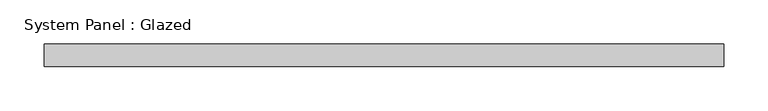
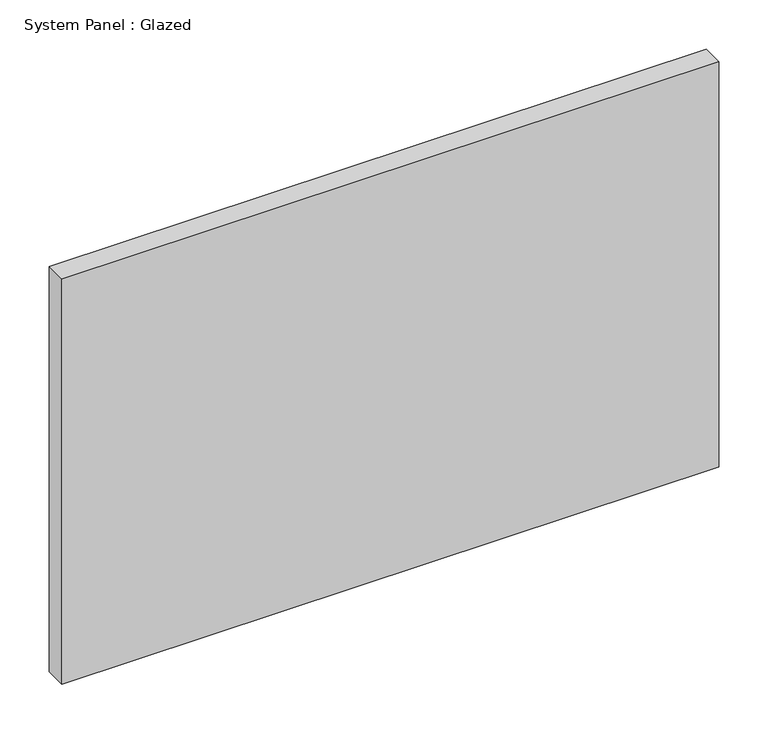
"""IFC4 building model written with IfcOpenShell, lengths in millimetres: plate geometry, System Panel : Glazed."""

from ifc_helpers import new_model, si_unit, origin, origin_with_axes, place, context, project, spatial, polyline, outline, extrude, source, transform, mapped, element, save


def system_panel_glazed_bfd0fd53(model_context):
    return source(origin(), model_context, "Body", "SweptSolid", [
        extrude(outline(polyline([(383.50825, 19.05), (-383.50825, 19.05), (-383.50825, 44.45), (383.50825, 44.45), (383.50825, 19.05)])), origin_with_axes(), (0.0, 0.0, 1.0), 500.761),
    ])


if __name__ == "__main__":
    model = new_model("IFC4")
    model_context = context("Model", 3, world=origin())
    ifc_project = project(units=[si_unit("LENGTHUNIT", "METRE", prefix="MILLI")], contexts=[model_context])
    site = spatial("IfcSite", under=ifc_project)
    building = spatial("IfcBuilding", under=site)
    placement = place(None, origin())
    system_panel_glazed_shape = system_panel_glazed_bfd0fd53(model_context)
    element("IfcPlate", 1, ObjectType="System Panel : Glazed", at=placement, inside=building, context=model_context, shape_type="MappedRepresentation", body=[
        mapped(system_panel_glazed_shape, transform((0.0, 0.0, 0.0), x_axis=(1.0, 0.0, 0.0), y_axis=(0.0, 1.0, 0.0), z_axis=(0.0, 0.0, 1.0))),
    ])
    save(model, "model.ifc")

# Revit data of these elements
# Type "System Panel : Glazed"
#   Construction Type Id = "GSP4R"
#   Analytic Construction = "1/8 in Pilkington single glazing"
#   Visual Light Transmittance = 0.9
#   Solar Heat Gain Coefficient = 0.86
#   Heat Transfer Coefficient (U) = 1.18115 BTU/(h·ft²·°F)
#   Define Thermal Properties by = 1
# Element 1 (IfcPlate, "System Panel : Glazed")
#   Materials on its faces: "Glass"
# Materials
#   "Glass": class "Glass", colour RGB 0 128 192, transparency 0.75, Description = "Soda Lime Glass", Cost = 0
